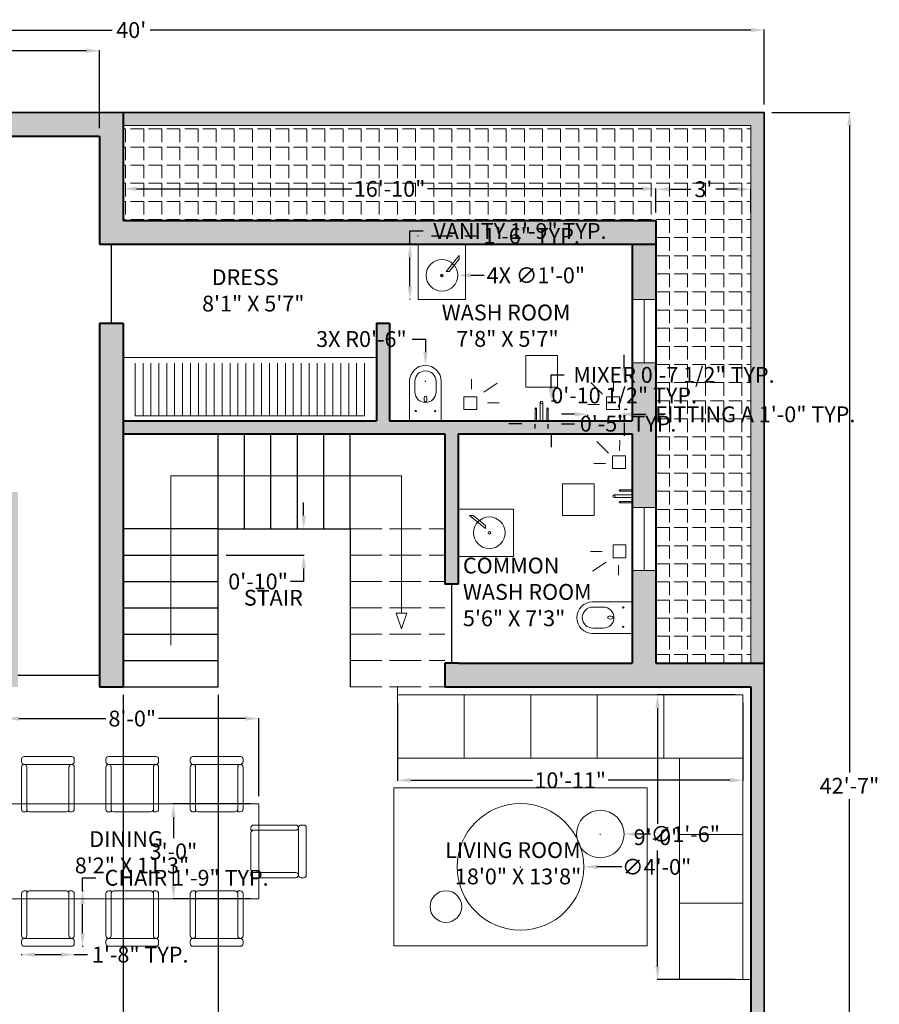
# Model space of a CAD drawing. Units: inches. Extents: x 242 to 808, y 202 to 873.
# Tile 3 of 3: x 482 to 808, y 500 to 873. Entities that reach past the tile are written whole.
import ezdxf

# ---------------------------------------------------------------- set-up
doc = ezdxf.new("R2010")
doc.units = ezdxf.units.IN
doc.header["$MEASUREMENT"] = 0
doc.linetypes.add('ACAD_ISO02W100', pattern=[15, 12, -3])
for name, color, linetype, lineweight in [('A-ANNO-DIMS', 2, 'Continuous', 18), ('A-ANNO-SYMB', 7, 'Continuous', 18), ('A-AREA-IDEN', 7, 'Continuous', 25), ('A-DOOR', 3, 'Continuous', 25), ('A-FLOR-CASE', 8, 'Continuous', 20), ('A-FLOR-FIXT', 8, 'Continuous', 18), ('A-FLOR-STRS', 7, 'Continuous', 25), ('A-FLOR-STRS-OVHD', 8, 'ACAD_ISO02W100', 18), ('A-FURN', 8, 'Continuous', 18), ('A-GLAZ', 4, 'Continuous', 18), ('A-SITE-PVMT', 8, 'Continuous', 18), ('A-SITE-PVMT-PATT', 254, 'Continuous', 13), ('A-WALL', 7, 'Continuous', 40), ('A-WALL-PATT', 30, 'Continuous', 13), ('C-PROP', 7, 'Continuous', 35)]:
    doc.layers.add(name, color=color, linetype=linetype, lineweight=lineweight)
doc.styles.get("Standard").update_dxf_attribs({"font": 'arial.ttf'})
doc.dimstyles.get("Standard").update_dxf_attribs({"dimtxt": 6, "dimasz": 5, "dimexe": 0.18, "dimexo": 3, "dimgap": 2, "dimtad": 0, "dimtih": 1, "dimtoh": 1, "dimdec": 0, "dimzin": 0, "dimdsep": 46, "dimlunit": 3, "dimtxsty": 'Standard', "dimcen": 0.09, "dimadec": 0, "dimazin": 0, "dimtfac": 1, "dimtdec": 0, "dimtofl": 0, "dimtmove": 0, "dimatfit": 3, "dimfxl": 1, "dimtolj": 1, "dimtzin": 0, "dimarcsym": 0})

# ---------------------------------------------------------------- blocks, each defined once
blk = doc.blocks.new('*U1')
blk.add_line((0, 0), (0, 20))
blk = doc.blocks.new('*U2')
at = {"layer": 'A-FLOR-CASE', "color": 0, "linetype": 'ByBlock', "lineweight": -2, "transparency": 16777216, "rotation": 90}
for p in [(883.16, 754.75), (883.16, 751.75), (883.16, 748.75), (883.16, 745.75), (883.16, 742.75), (883.16, 739.75), (883.16, 736.75), (883.16, 733.75), (883.16, 730.75), (883.16, 727.75), (883.16, 724.75), (883.16, 721.75), (883.16, 718.75), (883.16, 715.75), (883.16, 712.75), (883.16, 709.75), (883.16, 706.75), (883.16, 703.75), (883.16, 700.75), (883.16, 697.75), (883.16, 694.75), (883.16, 691.75), (883.16, 688.75), (883.16, 685.75), (883.16, 682.75), (883.16, 679.75), (883.16, 676.75), (883.16, 673.75), (883.16, 670.75), (883.16, 667.75)]:
    blk.add_blockref('*U1', p, dxfattribs=at)
blk = doc.blocks.new('*D5')
at = {"layer": 'A-ANNO-DIMS', "color": 0, "lineweight": -2, "transparency": 16777216}
for p, q in [((723.66, 800.15), (723.66, 809.17)), ((728.66, 808.99), (736.91, 808.99)), ((754.66, 808.99), (746.42, 808.99)), ((759.66, 800.15), (759.66, 809.17))]:
    blk.add_line(p, q, dxfattribs=at)
at = {"layer": 'A-ANNO-DIMS', "color": 0, "transparency": 16777216}
for points in [[(728.66, 809.82), (728.66, 808.16), (723.66, 808.99)], [(754.66, 809.82), (754.66, 808.16), (759.66, 808.99)]]:
    blk.add_solid(points, dxfattribs=at)
at = {"layer": 'Defpoints', "color": 0, "transparency": 16777216}
for p in [(759.66, 808.99), (723.66, 797.15), (759.66, 797.15)]:
    blk.add_point(p, dxfattribs=at)
at = {"layer": 'A-ANNO-DIMS', "color": 0, "transparency": 16777216, "insert": (741.66, 808.99), "char_height": 6, "attachment_point": 5}
blk.add_mtext("\\A1;3'", dxfattribs=at)
blk = doc.blocks.new('*D6')
at = {"layer": 'A-ANNO-DIMS', "color": 0, "lineweight": -2, "transparency": 16777216}
for p, q in [((521.66, 800.15), (521.66, 809.31)), ((526.66, 809.13), (608.31, 809.13)), ((718.66, 809.13), (637.02, 809.13)), ((723.66, 800.15), (723.66, 809.31))]:
    blk.add_line(p, q, dxfattribs=at)
at = {"layer": 'A-ANNO-DIMS', "color": 0, "transparency": 16777216}
for points in [[(526.66, 809.97), (526.66, 808.3), (521.66, 809.13)], [(718.66, 809.97), (718.66, 808.3), (723.66, 809.13)]]:
    blk.add_solid(points, dxfattribs=at)
at = {"layer": 'Defpoints', "color": 0, "transparency": 16777216}
for p in [(521.66, 809.13), (521.66, 797.15), (723.66, 797.15)]:
    blk.add_point(p, dxfattribs=at)
at = {"layer": 'A-ANNO-DIMS', "color": 0, "transparency": 16777216, "insert": (622.66, 809.13), "char_height": 6, "attachment_point": 5}
blk.add_mtext('\\A1;16\'-10"', dxfattribs=at)
blk = doc.blocks.new('*D7')
at = {"layer": 'A-ANNO-DIMS', "color": 0, "lineweight": -2, "transparency": 16777216}
for p, q in [((284.66, 841.15), (284.66, 869.56)), ((289.66, 869.38), (517.45, 869.38)), ((759.66, 869.38), (531.88, 869.38)), ((764.66, 841.15), (764.66, 869.56))]:
    blk.add_line(p, q, dxfattribs=at)
at = {"layer": 'A-ANNO-DIMS', "color": 0, "transparency": 16777216}
for points in [[(289.66, 870.21), (289.66, 868.54), (284.66, 869.38)], [(759.66, 870.21), (759.66, 868.54), (764.66, 869.38)]]:
    blk.add_solid(points, dxfattribs=at)
at = {"layer": 'Defpoints', "color": 0, "transparency": 16777216}
for p in [(764.66, 869.38), (284.66, 838.15), (764.66, 838.15)]:
    blk.add_point(p, dxfattribs=at)
at = {"layer": 'A-ANNO-DIMS', "color": 0, "transparency": 16777216, "insert": (524.66, 869.38), "char_height": 6, "attachment_point": 5}
blk.add_mtext("\\A1;40'", dxfattribs=at)
blk = doc.blocks.new('DINING-CHAIR')
for p, q in [((2, 18), (2, 20)), ((3, 21), (17, 21)), ((18, 21), (18, 18)), ((19, 21), (18, 21)), ((18, 20), (18, 18)), ((20, 4), (20, 20)), ((1, 0), (10, 0)), ((10, 0), (19, 0))]:
    blk.add_line(p, q)
for points in [[(0, 1), (0, 2, -0.414214), (1, 3), (1, 3, 0.414214), (2, 4), (2, 21), (1, 21, 0.414214), (0, 20), (0, 4, 0.414214), (1, 3), (19, 3)], [(18, 18), (18, 4, 0.414214), (19, 3), (19, 3, -0.414214), (20, 2), (20, 1)]]:
    blk.add_lwpolyline(points, format="xyb")
for centre, start, end in [((3, 20), 90, 180), ((17, 20), 0, 90), ((19, 20), 0, 90), ((19, 4), 270, 0), ((1, 1), 180, 270), ((19, 1), 270, 0)]:
    blk.add_arc(centre, 1, start, end)
blk = doc.blocks.new('LAVATORY-VANITY')
for p, q in [((15.59, 16.67), (10.6, 10.67)), ((11.73, 10.63), (15.59, 15.35)), ((15.59, 16.67), (15.59, 15.35)), ((10.6, 10.67), (11.73, 10.63))]:
    blk.add_line(p, q)
blk.add_lwpolyline([(0, 21), (18, 21), (18, 0), (0, 0)], close=True)
for radius in [6, 0.5]:
    blk.add_circle((8.99, 9.16), radius)
blk = doc.blocks.new('WC-PAN')
for p, q in [((0, 15), (0, 0)), ((12, 0), (12, 15)), ((2, 14.93), (2, 10.93)), ((10, 14.93), (10, 10.93))]:
    blk.add_line(p, q)
for centre, radius, start, end in [((6, 15), 6, 0, 180), ((6, 14.93), 4, 0, 180), ((6, 10.93), 4, 180, 0)]:
    blk.add_arc(centre, radius, start, end)
blk.add_ellipse((6, 8.26), major_axis=(0, 1.09), ratio=0.500408)
blk = doc.blocks.new('SHOWER-MIXER')
for p, q in [((0, 4.4), (0, 0)), ((0.5, 4.4), (0.5, 0)), ((2, 6.9), (2, 0)), ((3, 6.9), (3, 0)), ((4.5, 4.4), (4.5, 0)), ((5, 4.4), (5, 0))]:
    blk.add_line(p, q)
for centre, radius in [((0.25, 4.65), 0.25), ((2.5, 6.9), 0.5), ((4.75, 4.65), 0.25)]:
    blk.add_circle(centre, radius)
blk = doc.blocks.new('BATH-FITTING-A')
for p, q in [((5.56, 5.86), (1.12, 10.3)), ((9.72, 6.87), (9.79, 10.74)), ((4.44, 1.91), (0, 1.91))]:
    blk.add_line(p, q)
blk.add_lwpolyline([(7.09, 4.89), (11.98, 4.89), (11.98, 0), (7.09, 0)], close=True)
blk = doc.blocks.new('BATH-FITTING-B')
for p, q in [((2.85, 7.76), (2.85, 11.5)), ((7.55, 6.61), (12.62, 10.02)), ((9.01, 2.54), (13.42, 2.54))]:
    blk.add_line(p, q)
blk.add_lwpolyline([(0, 4.89), (4.89, 4.89), (4.89, 0), (0, 0)], close=True)
blk = doc.blocks.new('WIN-24IN')
blk.add_line((4.5, 24), (4.5, 0))
blk.add_lwpolyline([(0, 24), (9, 24), (9, 0), (0, 0)], close=True)
blk = doc.blocks.new('DOOR-30IN-PLAN')
blk.add_line((0, 30), (0, 0))
blk = doc.blocks.new('BATH-FITTING-12IN-SQ')
blk.add_lwpolyline([(0, 12), (12, 12), (12, 0), (0, 0)], close=True)
blk = doc.blocks.new('*D25')
at = {"layer": 'A-ANNO-DIMS', "color": 0, "lineweight": -2, "transparency": 16777216}
for p, q in [((506.21, 542.76), (506.21, 547.76)), ((506.21, 547.76), (511.21, 547.76)), ((506.06, 542.76), (506.39, 542.76)), ((506.21, 526.76), (506.21, 537.76)), ((506.06, 521.76), (506.39, 521.76))]:
    blk.add_line(p, q, dxfattribs=at)
at = {"layer": 'A-ANNO-DIMS', "color": 0, "transparency": 16777216}
for points in [[(505.38, 537.76), (507.05, 537.76), (506.21, 542.76)], [(505.38, 526.76), (507.05, 526.76), (506.21, 521.76)]]:
    blk.add_solid(points, dxfattribs=at)
at = {"layer": 'Defpoints', "color": 0, "transparency": 16777216}
for p in [(503.06, 542.76), (506.21, 542.76), (503.06, 521.76)]:
    blk.add_point(p, dxfattribs=at)
at = {"layer": 'A-ANNO-DIMS', "color": 0, "transparency": 16777216, "insert": (545.67, 547.76), "char_height": 6, "attachment_point": 5}
blk.add_mtext('\\A1;CHAIR 1\'-9" TYP.', dxfattribs=at)
blk = doc.blocks.new('*D26')
at = {"layer": 'A-ANNO-DIMS', "color": 0, "lineweight": -2, "transparency": 16777216}
for p, q in [((483.06, 518.76), (483.06, 518.43)), ((488.06, 518.61), (498.06, 518.61)), ((503.06, 518.76), (503.06, 518.43)), ((503.06, 518.61), (508.06, 518.61))]:
    blk.add_line(p, q, dxfattribs=at)
at = {"layer": 'A-ANNO-DIMS', "color": 0, "transparency": 16777216}
for points in [[(488.06, 519.44), (488.06, 517.77), (483.06, 518.61)], [(498.06, 519.44), (498.06, 517.77), (503.06, 518.61)]]:
    blk.add_solid(points, dxfattribs=at)
at = {"layer": 'Defpoints', "color": 0, "transparency": 16777216}
for p in [(483.06, 521.76), (503.06, 521.76), (503.06, 518.61)]:
    blk.add_point(p, dxfattribs=at)
at = {"layer": 'A-ANNO-DIMS', "color": 0, "transparency": 16777216, "insert": (528.07, 518.61), "char_height": 6, "attachment_point": 5}
blk.add_mtext('\\A1;1\'-8" TYP.', dxfattribs=at)
blk = doc.blocks.new('*D27')
at = {"layer": 'A-ANNO-DIMS', "color": 0, "lineweight": -2, "transparency": 16777216}
for p, q in [((630.35, 788.15), (630.35, 793.15)), ((630.35, 793.15), (635.35, 793.15)), ((630.5, 788.15), (630.17, 788.15)), ((630.35, 772.15), (630.35, 783.15)), ((630.5, 767.15), (630.17, 767.15))]:
    blk.add_line(p, q, dxfattribs=at)
at = {"layer": 'A-ANNO-DIMS', "color": 0, "transparency": 16777216}
for points in [[(629.51, 783.15), (631.18, 783.15), (630.35, 788.15)], [(629.51, 772.15), (631.18, 772.15), (630.35, 767.15)]]:
    blk.add_solid(points, dxfattribs=at)
at = {"layer": 'Defpoints', "color": 0, "transparency": 16777216}
for p in [(630.35, 788.15), (633.5, 788.15), (633.5, 767.15)]:
    blk.add_point(p, dxfattribs=at)
at = {"layer": 'A-ANNO-DIMS', "color": 0, "transparency": 16777216, "insert": (672.09, 793.15), "char_height": 6, "attachment_point": 5}
blk.add_mtext('\\A1;VANITY 1\'-9" TYP.', dxfattribs=at)
blk = doc.blocks.new('*D28')
at = {"layer": 'A-ANNO-DIMS', "color": 0, "lineweight": -2, "transparency": 16777216}
for p, q in [((633.5, 791.15), (633.5, 791.48)), ((638.5, 791.3), (646.5, 791.3)), ((651.5, 791.15), (651.5, 791.48)), ((651.5, 791.3), (656.5, 791.3))]:
    blk.add_line(p, q, dxfattribs=at)
at = {"layer": 'A-ANNO-DIMS', "color": 0, "transparency": 16777216}
for points in [[(638.5, 792.14), (638.5, 790.47), (633.5, 791.3)], [(646.5, 792.14), (646.5, 790.47), (651.5, 791.3)]]:
    blk.add_solid(points, dxfattribs=at)
at = {"layer": 'Defpoints', "color": 0, "transparency": 16777216}
for p in [(651.5, 791.3), (633.5, 788.15), (651.5, 788.15)]:
    blk.add_point(p, dxfattribs=at)
at = {"layer": 'A-ANNO-DIMS', "color": 0, "transparency": 16777216, "insert": (676.5, 791.3), "char_height": 6, "attachment_point": 5}
blk.add_mtext('\\A1;1\'-6" TYP.', dxfattribs=at)
blk = doc.blocks.new('*D31')
at = {"layer": 'A-ANNO-DIMS', "color": 0, "lineweight": -2, "transparency": 16777216}
for p, q in [((683.92, 733.55), (683.92, 738.55)), ((683.92, 738.55), (688.92, 738.55)), ((685.81, 728.55), (684.1, 728.55)), ((685.81, 721.15), (684.1, 721.15)), ((683.92, 716.15), (683.92, 711.15))]:
    blk.add_line(p, q, dxfattribs=at)
at = {"layer": 'A-ANNO-DIMS', "color": 0, "transparency": 16777216}
for points in [[(683.08, 733.55), (684.75, 733.55), (683.92, 728.55)], [(683.08, 716.15), (684.75, 716.15), (683.92, 721.15)]]:
    blk.add_solid(points, dxfattribs=at)
at = {"layer": 'Defpoints', "color": 0, "transparency": 16777216}
for p in [(682.81, 728.55), (683.92, 728.55), (682.81, 721.15)]:
    blk.add_point(p, dxfattribs=at)
at = {"layer": 'A-ANNO-DIMS', "color": 0, "transparency": 16777216, "insert": (730.5, 738.55), "char_height": 6, "attachment_point": 5}
blk.add_mtext('\\A1;MIXER 0\'-7 1/2" TYP.', dxfattribs=at)
blk = doc.blocks.new('*D32')
at = {"layer": 'A-ANNO-DIMS', "color": 0, "lineweight": -2, "transparency": 16777216}
for p, q in [((672.81, 720.04), (667.81, 720.04)), ((677.81, 718.15), (677.81, 719.86)), ((682.81, 718.15), (682.81, 719.86)), ((687.81, 720.04), (692.81, 720.04))]:
    blk.add_line(p, q, dxfattribs=at)
at = {"layer": 'A-ANNO-DIMS', "color": 0, "transparency": 16777216}
for points in [[(672.81, 720.88), (672.81, 719.21), (677.81, 720.04)], [(687.81, 720.88), (687.81, 719.21), (682.81, 720.04)]]:
    blk.add_solid(points, dxfattribs=at)
at = {"layer": 'Defpoints', "color": 0, "transparency": 16777216}
for p in [(677.81, 721.15), (682.81, 721.15), (682.81, 720.04)]:
    blk.add_point(p, dxfattribs=at)
at = {"layer": 'A-ANNO-DIMS', "color": 0, "transparency": 16777216, "insert": (713.1, 720.04), "char_height": 6, "attachment_point": 5}
blk.add_mtext('\\A1;0\'-5" TYP.', dxfattribs=at)
blk = doc.blocks.new('*D33')
at = {"layer": 'A-ANNO-DIMS', "color": 0, "lineweight": -2, "transparency": 16777216}
for p, q in [((692.82, 723.59), (687.82, 723.59)), ((697.82, 722.39), (697.82, 723.41)), ((709.8, 722.39), (709.8, 723.41)), ((714.8, 723.59), (719.8, 723.59))]:
    blk.add_line(p, q, dxfattribs=at)
at = {"layer": 'A-ANNO-DIMS', "color": 0, "transparency": 16777216}
for points in [[(692.82, 724.43), (692.82, 722.76), (697.82, 723.59)], [(714.8, 724.43), (714.8, 722.76), (709.8, 723.59)]]:
    blk.add_solid(points, dxfattribs=at)
at = {"layer": 'Defpoints', "color": 0, "transparency": 16777216}
for p in [(697.82, 725.39), (709.8, 725.39), (709.8, 723.59)]:
    blk.add_point(p, dxfattribs=at)
at = {"layer": 'A-ANNO-DIMS', "color": 0, "transparency": 16777216, "insert": (761.33, 723.59), "char_height": 6, "attachment_point": 5}
blk.add_mtext('\\A1;FITTING A 1\'-0" TYP.', dxfattribs=at)
blk = doc.blocks.new('*D34')
at = {"layer": 'A-ANNO-DIMS', "color": 0, "lineweight": -2, "transparency": 16777216}
for p, q in [((711.6, 741.13), (711.6, 746.13)), ((712.8, 736.13), (711.78, 736.13)), ((712.8, 725.39), (711.78, 725.39)), ((711.6, 720.39), (711.6, 715.39))]:
    blk.add_line(p, q, dxfattribs=at)
at = {"layer": 'A-ANNO-DIMS', "color": 0, "transparency": 16777216}
for points in [[(710.76, 741.13), (712.43, 741.13), (711.6, 736.13)], [(710.76, 720.39), (712.43, 720.39), (711.6, 725.39)]]:
    blk.add_solid(points, dxfattribs=at)
at = {"layer": 'Defpoints', "color": 0, "transparency": 16777216}
for p in [(709.8, 736.13), (711.6, 736.13), (709.8, 725.39)]:
    blk.add_point(p, dxfattribs=at)
at = {"layer": 'A-ANNO-DIMS', "color": 0, "transparency": 16777216, "insert": (711.6, 730.76), "char_height": 6, "attachment_point": 5}
blk.add_mtext('\\A1;0\'-10 1/2" TYP.', dxfattribs=at)
blk = doc.blocks.new('*D43')
at = {"layer": 'A-ANNO-DIMS', "color": 0, "lineweight": -2, "transparency": 16777216}
for p, q in [((334.66, 832.15), (334.66, 861.73)), ((339.66, 861.55), (409.31, 861.55)), ((507.66, 861.55), (438.02, 861.55)), ((512.66, 832.15), (512.66, 861.73))]:
    blk.add_line(p, q, dxfattribs=at)
at = {"layer": 'A-ANNO-DIMS', "color": 0, "transparency": 16777216}
for points in [[(339.66, 862.39), (339.66, 860.72), (334.66, 861.55)], [(507.66, 862.39), (507.66, 860.72), (512.66, 861.55)]]:
    blk.add_solid(points, dxfattribs=at)
at = {"layer": 'Defpoints', "color": 0, "transparency": 16777216}
for p in [(512.66, 861.55), (334.66, 829.15), (512.66, 829.15)]:
    blk.add_point(p, dxfattribs=at)
at = {"layer": 'A-ANNO-DIMS', "color": 0, "transparency": 16777216, "insert": (423.66, 861.55), "char_height": 6, "attachment_point": 5}
blk.add_mtext('\\A1;14\'-10"', dxfattribs=at)
blk = doc.blocks.new('*D47')
at = {"layer": 'A-ANNO-DIMS', "color": 0, "lineweight": -2, "transparency": 16777216}
for p, q in [((521.66, 617.15), (521.66, 205.57)), ((557.66, 617.15), (557.66, 205.57)), ((526.66, 205.75), (529.69, 205.75)), ((552.66, 205.75), (549.64, 205.75))]:
    blk.add_line(p, q, dxfattribs=at)
at = {"layer": 'A-ANNO-DIMS', "color": 0, "transparency": 16777216}
for points in [[(526.66, 206.59), (526.66, 204.92), (521.66, 205.75)], [(552.66, 206.59), (552.66, 204.92), (557.66, 205.75)]]:
    blk.add_solid(points, dxfattribs=at)
at = {"layer": 'Defpoints', "color": 0, "transparency": 16777216}
for p in [(521.66, 620.15), (557.66, 620.15), (557.66, 205.75)]:
    blk.add_point(p, dxfattribs=at)
at = {"layer": 'A-ANNO-DIMS', "color": 0, "transparency": 16777216, "insert": (539.66, 205.75), "char_height": 6, "attachment_point": 5}
blk.add_mtext('\\A1;3\'-0"', dxfattribs=at)
blk = doc.blocks.new('*D48')
at = {"layer": 'A-ANNO-DIMS', "color": 0, "lineweight": -2, "transparency": 16777216}
for p, q in [((767.66, 838.15), (797.24, 838.15)), ((797.06, 833.15), (797.06, 587.67)), ((797.06, 332.15), (797.06, 577.64)), ((546.66, 327.15), (797.24, 327.15))]:
    blk.add_line(p, q, dxfattribs=at)
at = {"layer": 'A-ANNO-DIMS', "color": 0, "transparency": 16777216}
for points in [[(796.23, 833.15), (797.9, 833.15), (797.06, 838.15)], [(796.23, 332.15), (797.9, 332.15), (797.06, 327.15)]]:
    blk.add_solid(points, dxfattribs=at)
at = {"layer": 'Defpoints', "color": 0, "transparency": 16777216}
for p in [(764.66, 838.15), (797.06, 838.15), (543.66, 327.15)]:
    blk.add_point(p, dxfattribs=at)
at = {"layer": 'A-ANNO-DIMS', "color": 0, "transparency": 16777216, "insert": (797.06, 582.65), "char_height": 6, "attachment_point": 5}
blk.add_mtext('\\A1;42\'-7"', dxfattribs=at)
blk = doc.blocks.new('*D50')
at = {"layer": 'A-ANNO-DIMS', "color": 0, "lineweight": -2, "transparency": 16777216}
for p, q in [((477.06, 578.76), (477.06, 608.34)), ((482.06, 608.16), (515.08, 608.16)), ((568.06, 608.16), (535.04, 608.16)), ((573.06, 578.76), (573.06, 608.34))]:
    blk.add_line(p, q, dxfattribs=at)
at = {"layer": 'A-ANNO-DIMS', "color": 0, "transparency": 16777216}
for points in [[(482.06, 608.99), (482.06, 607.32), (477.06, 608.16)], [(568.06, 608.99), (568.06, 607.32), (573.06, 608.16)]]:
    blk.add_solid(points, dxfattribs=at)
at = {"layer": 'Defpoints', "color": 0, "transparency": 16777216}
for p in [(573.06, 608.16), (477.06, 575.76), (573.06, 575.76)]:
    blk.add_point(p, dxfattribs=at)
at = {"layer": 'A-ANNO-DIMS', "color": 0, "transparency": 16777216, "insert": (525.06, 608.16), "char_height": 6, "attachment_point": 5}
blk.add_mtext('\\A1;8\'-0"', dxfattribs=at)
blk = doc.blocks.new('*D51')
at = {"layer": 'A-ANNO-DIMS', "color": 0, "lineweight": -2, "transparency": 16777216}
for p, q in [((570.06, 575.76), (540.48, 575.76)), ((540.66, 570.76), (540.66, 562.82)), ((540.66, 544.76), (540.66, 552.69)), ((570.06, 539.76), (540.48, 539.76))]:
    blk.add_line(p, q, dxfattribs=at)
at = {"layer": 'A-ANNO-DIMS', "color": 0, "transparency": 16777216}
for points in [[(539.83, 570.76), (541.5, 570.76), (540.66, 575.76)], [(539.83, 544.76), (541.5, 544.76), (540.66, 539.76)]]:
    blk.add_solid(points, dxfattribs=at)
at = {"layer": 'Defpoints', "color": 0, "transparency": 16777216}
for p in [(540.66, 575.76), (573.06, 575.76), (573.06, 539.76)]:
    blk.add_point(p, dxfattribs=at)
at = {"layer": 'A-ANNO-DIMS', "color": 0, "transparency": 16777216, "insert": (540.66, 557.76), "char_height": 6, "attachment_point": 5}
blk.add_mtext('\\A1;3\'-0"', dxfattribs=at)
blk = doc.blocks.new('*D52')
at = {"layer": 'A-ANNO-DIMS', "color": 0, "lineweight": -2, "transparency": 16777216}
for p, q in [((590.06, 685.15), (590.06, 690.15)), ((560.66, 680.15), (590.24, 680.15)), ((560.66, 670.15), (590.24, 670.15)), ((590.06, 665.15), (590.06, 660.15)), ((590.06, 660.15), (585.06, 660.15))]:
    blk.add_line(p, q, dxfattribs=at)
at = {"layer": 'A-ANNO-DIMS', "color": 0, "transparency": 16777216}
for points in [[(589.23, 685.15), (590.9, 685.15), (590.06, 680.15)], [(589.23, 665.15), (590.9, 665.15), (590.06, 670.15)]]:
    blk.add_solid(points, dxfattribs=at)
at = {"layer": 'Defpoints', "color": 0, "transparency": 16777216}
for p in [(557.66, 680.15), (557.66, 670.15), (590.06, 670.15)]:
    blk.add_point(p, dxfattribs=at)
at = {"layer": 'A-ANNO-DIMS', "color": 0, "transparency": 16777216, "insert": (572.76, 660.15), "char_height": 6, "attachment_point": 5}
blk.add_mtext('\\A1;0\'-10"', dxfattribs=at)
blk = doc.blocks.new('*D56')
at = {"layer": 'A-ANNO-DIMS', "color": 0, "lineweight": -2, "transparency": 16777216}
for p, q in [((625.66, 614.15), (625.66, 584.57)), ((756.66, 614.15), (756.66, 584.57)), ((630.66, 584.75), (676.81, 584.75)), ((751.66, 584.75), (705.52, 584.75))]:
    blk.add_line(p, q, dxfattribs=at)
at = {"layer": 'A-ANNO-DIMS', "color": 0, "transparency": 16777216}
for points in [[(630.66, 585.59), (630.66, 583.92), (625.66, 584.75)], [(751.66, 585.59), (751.66, 583.92), (756.66, 584.75)]]:
    blk.add_solid(points, dxfattribs=at)
at = {"layer": 'Defpoints', "color": 0, "transparency": 16777216}
for p in [(625.66, 617.15), (756.66, 617.15), (625.66, 584.75)]:
    blk.add_point(p, dxfattribs=at)
at = {"layer": 'A-ANNO-DIMS', "color": 0, "transparency": 16777216, "insert": (691.16, 584.75), "char_height": 6, "attachment_point": 5}
blk.add_mtext('\\A1;10\'-11"', dxfattribs=at)
blk = doc.blocks.new('*D57')
at = {"layer": 'A-ANNO-DIMS', "color": 0, "lineweight": -2, "transparency": 16777216}
for p, q in [((753.66, 617.15), (724.08, 617.15)), ((724.26, 612.15), (724.26, 568.22)), ((724.26, 514.15), (724.26, 558.09)), ((753.66, 509.15), (724.08, 509.15))]:
    blk.add_line(p, q, dxfattribs=at)
at = {"layer": 'A-ANNO-DIMS', "color": 0, "transparency": 16777216}
for points in [[(723.43, 612.15), (725.1, 612.15), (724.26, 617.15)], [(723.43, 514.15), (725.1, 514.15), (724.26, 509.15)]]:
    blk.add_solid(points, dxfattribs=at)
at = {"layer": 'Defpoints', "color": 0, "transparency": 16777216}
for p in [(724.26, 617.15), (756.66, 617.15), (756.66, 509.15)]:
    blk.add_point(p, dxfattribs=at)
at = {"layer": 'A-ANNO-DIMS', "color": 0, "transparency": 16777216, "insert": (724.26, 563.15), "char_height": 6, "attachment_point": 5}
blk.add_mtext('\\A1;9\'-0"', dxfattribs=at)
blk = doc.blocks.new('*D58')
at = {"layer": 'A-ANNO-DIMS', "color": 0, "lineweight": -2, "transparency": 16777216}
for p, q in [((672.19, 551.88), (672.37, 551.88)), ((672.28, 551.79), (672.28, 551.97)), ((710.68, 551.88), (701.28, 551.88))]:
    blk.add_line(p, q, dxfattribs=at)
at = {"layer": 'A-ANNO-DIMS', "color": 0, "transparency": 16777216}
blk.add_solid([(701.28, 552.72), (701.28, 551.05), (696.28, 551.88)], dxfattribs=at)
at = {"layer": 'Defpoints', "color": 0, "transparency": 16777216}
for p in [(648.28, 551.88), (696.28, 551.88)]:
    blk.add_point(p, dxfattribs=at)
at = {"layer": 'A-ANNO-DIMS', "color": 0, "transparency": 16777216, "insert": (723.91, 551.88), "char_height": 6, "attachment_point": 5}
blk.add_mtext('\\A1;∅4\'-0"', dxfattribs=at)
blk = doc.blocks.new('*D59')
at = {"layer": 'A-ANNO-DIMS', "color": 0, "lineweight": -2, "transparency": 16777216}
for p, q in [((702.48, 564.33), (702.66, 564.33)), ((702.57, 564.24), (702.57, 564.42)), ((721.57, 564.33), (716.57, 564.33))]:
    blk.add_line(p, q, dxfattribs=at)
at = {"layer": 'A-ANNO-DIMS', "color": 0, "transparency": 16777216}
blk.add_solid([(716.57, 565.16), (716.57, 563.5), (711.57, 564.33)], dxfattribs=at)
at = {"layer": 'Defpoints', "color": 0, "transparency": 16777216}
for p in [(693.57, 564.33), (711.57, 564.33)]:
    blk.add_point(p, dxfattribs=at)
at = {"layer": 'A-ANNO-DIMS', "color": 0, "transparency": 16777216, "insert": (734.81, 564.33), "char_height": 6, "attachment_point": 5}
blk.add_mtext('\\A1;∅1\'-6"', dxfattribs=at)
blk = doc.blocks.new('*D60')
at = {"layer": 'A-ANNO-DIMS', "color": 0, "lineweight": -2, "transparency": 16777216}
for p, q in [((642.39, 776.31), (642.57, 776.31)), ((642.48, 776.22), (642.48, 776.4)), ((658.48, 776.31), (653.48, 776.31))]:
    blk.add_line(p, q, dxfattribs=at)
at = {"layer": 'A-ANNO-DIMS', "color": 0, "transparency": 16777216}
blk.add_solid([(653.48, 777.15), (653.48, 775.48), (648.48, 776.31)], dxfattribs=at)
at = {"layer": 'Defpoints', "color": 0, "transparency": 16777216}
for p in [(636.48, 776.31), (648.48, 776.31)]:
    blk.add_point(p, dxfattribs=at)
at = {"layer": 'A-ANNO-DIMS', "color": 0, "transparency": 16777216, "insert": (678.13, 776.31), "char_height": 6, "attachment_point": 5}
blk.add_mtext('\\A1;4X ∅1\'-0"', dxfattribs=at)
blk = doc.blocks.new('*D61')
at = {"layer": 'A-ANNO-DIMS', "color": 0, "lineweight": -2, "transparency": 16777216}
for p, q in [((631.25, 752.15), (636.25, 752.15)), ((636.25, 752.15), (636.25, 747.15)), ((636.16, 736.15), (636.34, 736.15)), ((636.25, 736.06), (636.25, 736.24))]:
    blk.add_line(p, q, dxfattribs=at)
at = {"layer": 'A-ANNO-DIMS', "color": 0, "transparency": 16777216}
blk.add_solid([(637.08, 747.15), (635.41, 747.15), (636.25, 742.15)], dxfattribs=at)
at = {"layer": 'Defpoints', "color": 0, "transparency": 16777216}
for p in [(636.25, 742.15), (636.25, 736.15)]:
    blk.add_point(p, dxfattribs=at)
at = {"layer": 'A-ANNO-DIMS', "color": 0, "transparency": 16777216, "insert": (611.96, 752.15), "char_height": 6, "attachment_point": 5}
blk.add_mtext('\\A1;3X R0\'-6"', dxfattribs=at)

msp = doc.modelspace()

# ---------------------------------------------------------------- hatches: boundary and pattern name
at = {"layer": 'A-SITE-PVMT-PATT'}
h = msp.add_hatch(dxfattribs=at)
h.set_pattern_fill('ANGLE', color=256, scale=25, angle=180)
h.set_pattern_definition([(180, (0, 0), (-8e-16, -6.875), [5, -1.875]), (270, (0, 0), (6.875, -1e-15), [5, -1.875])])
h.paths.add_polyline_path([(759.66, 833.15), (521.66, 833.15), (521.66, 797.15), (723.66, 797.15), (723.66, 629.15), (759.66, 629.15)])
h.paths.add_polyline_path([(737.05, 802.77), (746.32, 802.77), (746.32, 815.13), (737.05, 815.13)], flags=24)
h.paths.add_polyline_path([(607.9, 802.91), (636.91, 802.91), (636.91, 815.27), (607.9, 815.27)], flags=24)
at = {"layer": 'A-WALL-PATT'}
h = msp.add_hatch(color=256, dxfattribs=at)
h.dxf.hatch_style = 1
h.paths.add_polyline_path([(521.66, 838.15), (325.66, 838.15), (325.66, 789.05), (334.66, 789.05), (334.66, 829.15), (512.66, 829.15), (512.66, 788.15), (714.66, 788.15), (723.66, 788.15), (723.66, 797.15), (521.66, 797.15)])
h.paths.add_polyline_path([(764.66, 838.15), (521.66, 838.15), (521.66, 833.15), (759.66, 833.15), (759.66, 629.15), (764.66, 629.15)])
h.paths.add_polyline_path([(723.66, 788.15), (714.66, 788.15), (714.66, 767.17), (723.66, 767.17)], flags=17)
h.paths.add_polyline_path([(723.66, 743.17), (714.66, 743.17), (714.66, 721.15), (622.66, 721.15), (622.66, 758.15), (617.66, 758.15), (617.66, 721.15), (521.66, 721.15), (521.66, 716.15), (643.66, 716.15), (643.66, 659.15), (648.66, 659.15), (648.66, 716.15), (714.66, 716.15), (714.66, 688.28), (723.66, 688.28)], flags=17)
h.paths.add_polyline_path([(764.66, 629.15), (759.66, 629.15), (723.66, 629.15), (723.66, 664.28), (714.66, 664.28), (714.66, 629.15), (648.66, 629.15), (643.66, 629.15), (643.66, 620.15), (759.66, 620.15), (759.66, 403.15), (759.66, 398.15), (759.66, 238.15), (764.66, 238.15)])
h.paths.add_polyline_path([(521.66, 758.15), (512.66, 758.15), (512.66, 620.15), (521.66, 620.15)])
h.paths.add_polyline_path([(481.66, 694.15), (334.66, 694.15), (334.66, 689.15), (476.66, 689.15), (476.66, 629.15), (481.66, 629.15)])
h.paths.add_polyline_path([(334.66, 741.05), (325.66, 741.05), (325.66, 675.31), (334.66, 675.31), (334.66, 689.15), (334.66, 694.15)], flags=17)
h.paths.add_polyline_path([(334.66, 651.31), (325.66, 651.31), (325.66, 629.15), (289.66, 629.15), (289.66, 838.15), (284.66, 838.15), (284.66, 620.15), (293.66, 620.15), (334.66, 620.15)])
h.paths.add_polyline_path([(293.66, 620.15), (284.66, 620.15), (284.66, 485.15), (293.66, 485.15)])
h.paths.add_polyline_path([(307.66, 485.15), (293.66, 485.15), (284.66, 485.15), (284.66, 238.15), (615.66, 238.15), (615.66, 243.15), (289.66, 243.15), (289.66, 480.15), (307.66, 480.15)])
h.paths.add_polyline_path([(373.66, 485.15), (355.66, 485.15), (355.66, 480.15), (373.66, 480.15)], flags=17)
h.paths.add_polyline_path([(445.66, 620.15), (440.66, 620.15), (440.66, 485.15), (373.66, 485.15), (373.66, 480.15), (373.66, 415.15), (410.66, 415.15), (410.66, 420.15), (378.66, 420.15), (378.66, 480.15), (440.66, 480.15), (440.66, 415.15), (445.66, 415.15)])
h.paths.add_polyline_path([(472.95, 336.15), (444.15, 336.15), (444.15, 327.15), (472.95, 327.15)], flags=17)
h.paths.add_polyline_path([(543.66, 485.15), (481.66, 485.15), (481.66, 480.15), (534.66, 480.15), (534.66, 336.15), (520.95, 336.15), (520.95, 327.15), (543.66, 327.15)], flags=17)
h.paths.add_polyline_path([(699.66, 456.15), (649.16, 456.15), (649.16, 451.15), (694.66, 451.15), (694.66, 398.15), (759.66, 398.15), (759.66, 403.15), (699.66, 403.15)], flags=17)
h.paths.add_polyline_path([(481.66, 629.15), (476.66, 629.15), (364.66, 629.15), (364.66, 620.15), (481.66, 620.15)])

# ---------------------------------------------------------------- linework, layer by layer
at = {"layer": 'A-ANNO-SYMB'}
for p, q in [((539.66, 640.15), (539.66, 700.21)), ((539.66, 700.21), (627.17, 700.21)), ((627.17, 700.21), (627.17, 648.16)), ((629.17, 648.16), (625.17, 648.16)), ((625.17, 648.16), (627.17, 642.16)), ((627.17, 642.16), (629.17, 648.16)), ((539.66, 640.15), (539.66, 635.98))]:
    msp.add_line(p, q, dxfattribs=at)
at = {"layer": 'A-DOOR'}
msp.add_line((481.66, 624.65), (512.66, 624.65), dxfattribs=at)
at = {"layer": 'A-FLOR-CASE'}
for p, q in [((521.66, 745.15), (617.66, 745.15)), ((613.14, 723.05), (526.14, 723.05))]:
    msp.add_line(p, q, dxfattribs=at)
at = {"layer": 'A-FLOR-FIXT'}
for centre in [(632.56, 724.85), (639.94, 724.85), (711.25, 650.35), (711.25, 642.96)]:
    msp.add_circle(centre, 0.25, dxfattribs=at)
at = {"layer": 'A-FLOR-STRS'}
for p, q in [((557.66, 680.15), (557.66, 716.15)), ((567.66, 680.15), (567.66, 716.15)), ((577.66, 680.15), (577.66, 716.15)), ((587.66, 680.15), (587.66, 716.15)), ((597.66, 680.15), (597.66, 716.15)), ((607.66, 680.15), (607.66, 716.15)), ((557.66, 680.15), (521.66, 680.15)), ((557.66, 620.15), (557.66, 680.15)), ((557.66, 680.15), (607.66, 680.15)), ((607.66, 680.15), (607.66, 620.15)), ((521.66, 670.15), (557.66, 670.15)), ((521.66, 660.15), (557.66, 660.15)), ((521.66, 650.15), (557.66, 650.15)), ((521.66, 640.15), (557.66, 640.15)), ((521.66, 630.15), (557.66, 630.15)), ((521.66, 620.15), (557.66, 620.15))]:
    msp.add_line(p, q, dxfattribs=at)
at = {"layer": 'A-FLOR-STRS-OVHD'}
for p, q in [((607.66, 680.15), (643.66, 680.15)), ((607.66, 670.15), (643.66, 670.15)), ((607.66, 660.15), (643.66, 660.15)), ((607.66, 650.15), (643.66, 650.15)), ((607.66, 640.15), (643.66, 640.15)), ((607.66, 630.15), (643.66, 630.15)), ((607.66, 620.15), (643.66, 620.15))]:
    msp.add_line(p, q, dxfattribs=at)
at = {"layer": 'A-FURN'}
for p, q in [((625.66, 620.15), (625.66, 593.15)), ((625.66, 617.15), (756.66, 617.15)), ((650.91, 593.15), (650.91, 617.15)), ((676.16, 593.15), (676.16, 617.15)), ((701.41, 593.15), (701.41, 617.15)), ((726.66, 593.15), (726.66, 617.15)), ((756.66, 617.15), (756.66, 509.15)), ((625.66, 593.15), (732.66, 593.15)), ((732.66, 593.15), (732.66, 509.15)), ((732.66, 593.15), (756.66, 593.15)), ((570.06, 566.76), (570.06, 565.76)), ((570.06, 565.76), (573.06, 565.76)), ((570.06, 550.76), (570.06, 564.76)), ((587.06, 567.76), (571.06, 567.76)), ((571.06, 565.76), (573.06, 565.76)), ((591.06, 557.76), (591.06, 566.76)), ((732.66, 564.15), (756.66, 564.15)), ((591.06, 548.76), (591.06, 557.76)), ((573.06, 549.76), (571.06, 549.76)), ((732.66, 538.15), (756.66, 538.15)), ((732.66, 509.15), (759.66, 509.15))]:
    msp.add_line(p, q, dxfattribs=at)
for points in [[(624.28, 581.88), (720.28, 581.88), (720.28, 521.88), (624.28, 521.88)], [(477.06, 575.76), (573.06, 575.76), (573.06, 539.76), (477.06, 539.76)]]:
    msp.add_lwpolyline(points, close=True, dxfattribs=at)
for points in [[(590.06, 547.76), (589.06, 547.76, -0.414214), (588.06, 548.76), (588.06, 548.76, 0.414214), (587.06, 549.76), (570.06, 549.76), (570.06, 548.76, 0.414214), (571.06, 547.76), (587.06, 547.76, 0.414214), (588.06, 548.76), (588.06, 566.76)], [(573.06, 565.76), (587.06, 565.76, 0.414214), (588.06, 566.76), (588.06, 566.76, -0.414214), (589.06, 567.76), (590.06, 567.76)]]:
    msp.add_lwpolyline(points, format="xyb", dxfattribs=at)
for centre, radius in [((672.28, 551.88), 24), ((702.57, 564.33), 9), ((643.99, 536.84), 6)]:
    msp.add_circle(centre, radius, dxfattribs=at)
for centre, start, end in [((571.06, 566.76), 90, 180), ((571.06, 564.76), 90, 180), ((587.06, 566.76), 0, 90), ((590.06, 566.76), 0, 90), ((571.06, 550.76), 180, 270), ((590.06, 548.76), 270, 0)]:
    msp.add_arc(centre, 1, start, end, dxfattribs=at)
at = {"layer": 'A-SITE-PVMT'}
for p, q in [((521.66, 833.15), (759.66, 833.15)), ((759.66, 833.15), (759.66, 629.15))]:
    msp.add_line(p, q, dxfattribs=at)
at = {"layer": 'A-WALL'}
for p, q in [((521.66, 838.15), (521.66, 797.15)), ((334.66, 829.15), (512.66, 829.15)), ((512.66, 829.15), (512.66, 788.15)), ((521.66, 797.15), (723.66, 797.15)), ((723.66, 797.15), (723.66, 629.15)), ((512.66, 788.15), (714.66, 788.15)), ((521.66, 788.15), (617.66, 788.15)), ((714.66, 788.15), (714.66, 721.15)), ((714.66, 788.15), (723.66, 788.15)), ((512.66, 758.15), (521.66, 758.15)), ((512.66, 758.15), (512.66, 620.15)), ((521.66, 758.15), (521.66, 620.15)), ((617.66, 758.15), (617.66, 721.15)), ((617.66, 758.15), (622.66, 758.15)), ((622.66, 758.15), (622.66, 721.15)), ((521.66, 721.15), (617.66, 721.15)), ((622.66, 721.15), (714.66, 721.15)), ((521.66, 716.15), (643.66, 716.15)), ((643.66, 716.15), (643.66, 659.15)), ((648.66, 716.15), (648.66, 659.15)), ((648.66, 716.15), (714.66, 716.15)), ((714.66, 716.15), (714.66, 629.15)), ((648.66, 659.15), (643.66, 659.15)), ((648.66, 629.15), (643.66, 629.15)), ((643.66, 629.15), (643.66, 620.15)), ((648.66, 629.15), (714.66, 629.15)), ((723.66, 629.15), (759.66, 629.15)), ((759.66, 629.15), (764.66, 629.15)), ((512.66, 620.15), (521.66, 620.15)), ((643.66, 620.15), (759.66, 620.15)), ((759.66, 620.15), (759.66, 403.15))]:
    msp.add_line(p, q, dxfattribs=at)
at = {"layer": 'C-PROP'}
for p, q in [((284.66, 838.15), (764.66, 838.15)), ((764.66, 838.15), (764.66, 238.15))]:
    msp.add_line(p, q, dxfattribs=at)

# ---------------------------------------------------------------- block references
at = {"layer": 'A-DOOR', "rotation": 180}
msp.add_blockref('DOOR-30IN-PLAN', (517.16, 788.15), dxfattribs=at)
at = {"layer": 'A-DOOR'}
msp.add_blockref('DOOR-30IN-PLAN', (646.16, 629.15), dxfattribs=at)
at = {"layer": 'A-FLOR-CASE', "rotation": 270}
msp.add_blockref('*U2', (-141.62, 1606.2), dxfattribs=at)
at = {"layer": 'A-FLOR-FIXT'}
for name, p in [('LAVATORY-VANITY', (633.5, 767.15)), ('BATH-FITTING-12IN-SQ', (674.31, 733.95)), ('WC-PAN', (630.25, 721.15)), ('BATH-FITTING-B', (650.82, 725.39)), ('BATH-FITTING-A', (697.82, 725.39)), ('SHOWER-MIXER', (677.81, 721.15)), ('BATH-FITTING-A', (700.12, 703.01))]:
    msp.add_blockref(name, p, dxfattribs=at)
for name, p, rotation in [('BATH-FITTING-12IN-SQ', (700.28, 685.18), 90.00000000000045), ('SHOWER-MIXER', (714.66, 689.99), 89.99999999999912), ('LAVATORY-VANITY', (669.66, 669.65), 90.00000000000028), ('BATH-FITTING-B', (712.28, 674.07), 180), ('WC-PAN', (714.66, 640.46), 89.9999999999989)]:
    msp.add_blockref(name, p, dxfattribs=dict(at, rotation=rotation))
at = {"layer": 'A-FURN', "extrusion": (0, 0, -1), "zscale": -1, "rotation": 180}
for p in [(-483.06, 593.76), (-515.06, 593.76), (-547.06, 593.76)]:
    msp.add_blockref('DINING-CHAIR', p, dxfattribs=at)
at = {"layer": 'A-FURN'}
for p in [(483.06, 521.76), (515.06, 521.76), (547.06, 521.76)]:
    msp.add_blockref('DINING-CHAIR', p, dxfattribs=at)
at = {"layer": 'A-GLAZ'}
for p in [(714.66, 743.17), (714.66, 664.28)]:
    msp.add_blockref('WIN-24IN', p, dxfattribs=at)

# ---------------------------------------------------------------- texts
at = {"layer": 'A-AREA-IDEN', "char_height": 6, "attachment_point": 1}
for s, insert in [('      DRESS\\P    8\'1" X 5\'7"', (544.19, 778.61)), ('WASH ROOM \\P   7\'8" X 5\'7"', (642.42, 765.22)), ('COMMON\\PWASH ROOM\\P5\'6" X 7\'3"', (650.46, 669.21)), ('STAIR', (567.37, 657)), ('   DINING \\P8\'2" X 11\'3"', (503.26, 565.43)), ('  LIVING ROOM\\P    18\'0" X 13\'8"', (640.09, 561.26))]:
    msp.add_mtext_dynamic_manual_height_columns(s, width=78.0144, gutter_width=1, heights=[0], dxfattribs=dict(at, insert=insert))

# ---------------------------------------------------------------- dimensions: what is measured, and where the dimension line sits
at = {"layer": 'A-ANNO-DIMS'}
for base, p1, p2, override, picture, middle in [((764.66, 869.38), (284.66, 838.15), (764.66, 838.15), {"dimclrd": 0, "dimclre": 0, "dimclrt": 0}, '*D7', (524.66, 869.38)), ((512.66, 861.55), (334.66, 829.15), (512.66, 829.15), {"dimdec": 1, "dimlfac": 1, "dimrnd": 0, "dimzin": 1, "dimdsep": 46, "dimlunit": 4, "dimfrac": 2}, '*D43', (423.66, 861.55)), ((521.66, 809.13), (723.66, 797.15), (521.66, 797.15), {"dimclrd": 0, "dimclre": 0, "dimclrt": 0}, '*D6', (622.66, 809.13)), ((759.66, 808.99), (723.66, 797.15), (759.66, 797.15), {"dimclrd": 0, "dimclre": 0, "dimclrt": 0}, '*D5', (741.66, 808.99)), ((557.66, 205.75), (521.66, 620.15), (557.66, 620.15), {"dimdec": 1, "dimlfac": 1, "dimrnd": 0, "dimzin": 1, "dimdsep": 46, "dimlunit": 4, "dimfrac": 2}, '*D47', (539.66, 205.75)), ((573.06, 608.16), (477.06, 575.76), (573.06, 575.76), {"dimdec": 1, "dimlfac": 1, "dimrnd": 0, "dimzin": 1, "dimdsep": 46, "dimlunit": 4, "dimfrac": 2}, '*D50', (525.06, 608.16))]:
    dim = msp.add_linear_dim(base=base, p1=p1, p2=p2, dimstyle='Standard', override=override, dxfattribs=at)
    dim.commit()
    dim.dimension.update_dxf_attribs({"geometry": picture, "text_midpoint": middle})
for base, p1, p2, angle, picture, middle in [((797.06, 838.15), (543.66, 327.15), (764.66, 838.15), 90, '*D48', (797.06, 582.65)), ((590.06, 670.15), (557.66, 680.15), (557.66, 670.15), 270, '*D52', (572.76, 660.15)), ((625.66, 584.75), (756.66, 617.15), (625.66, 617.15), 180, '*D56', (691.16, 584.75)), ((724.26, 617.15), (756.66, 509.15), (756.66, 617.15), 90, '*D57', (724.26, 563.15)), ((540.66, 575.76), (573.06, 539.76), (573.06, 575.76), 90, '*D51', (540.66, 557.76))]:
    dim = msp.add_linear_dim(base=base, p1=p1, p2=p2, angle=angle, dimstyle='Standard', override={"dimdec": 1, "dimlfac": 1, "dimrnd": 0, "dimzin": 1, "dimdsep": 46, "dimlunit": 4, "dimfrac": 2}, dxfattribs=at)
    dim.commit()
    dim.dimension.update_dxf_attribs({"geometry": picture, "text_midpoint": middle})
for base, p1, p2, text, picture, middle in [((630.35, 788.15), (633.5, 767.15), (633.5, 788.15), 'VANITY <> TYP.', '*D27', (672.09, 793.15)), ((683.92, 728.55), (682.81, 721.15), (682.81, 728.55), 'MIXER <> TYP.', '*D31', (730.5, 738.55)), ((711.6, 736.13), (709.8, 725.39), (709.8, 736.13), '<> TYP.', '*D34', (711.6, 730.76)), ((506.21, 542.76), (503.06, 521.76), (503.06, 542.76), 'CHAIR <> TYP.', '*D25', (545.67, 547.76))]:
    dim = msp.add_linear_dim(base=base, p1=p1, p2=p2, angle=90, text=text, dimstyle='Standard', override={"dimdec": 1, "dimlfac": 1, "dimrnd": 0, "dimzin": 1, "dimdsep": 46, "dimlunit": 4, "dimfrac": 2}, dxfattribs=at)
    dim.commit()
    dim.dimension.update_dxf_attribs({"geometry": picture, "text_midpoint": middle})
for base, p1, p2, text, picture, middle in [((651.5, 791.3), (633.5, 788.15), (651.5, 788.15), '<> TYP.', '*D28', (676.5, 791.3)), ((709.8, 723.59), (697.82, 725.39), (709.8, 725.39), 'FITTING A <> TYP.', '*D33', (761.33, 723.59)), ((682.81, 720.04), (677.81, 721.15), (682.81, 721.15), '<> TYP.', '*D32', (713.1, 720.04)), ((503.06, 518.61), (483.06, 521.76), (503.06, 521.76), '<> TYP.', '*D26', (528.07, 518.61))]:
    dim = msp.add_linear_dim(base=base, p1=p1, p2=p2, text=text, dimstyle='Standard', override={"dimdec": 1, "dimlfac": 1, "dimrnd": 0, "dimzin": 1, "dimdsep": 46, "dimlunit": 4, "dimfrac": 2}, dxfattribs=at)
    dim.commit()
    dim.dimension.update_dxf_attribs({"geometry": picture, "text_midpoint": middle})
dim = msp.add_diameter_dim_2p(p1=(636.48, 776.31), p2=(648.48, 776.31), text='4X <>', dimstyle='Standard', override={"dimdec": 1, "dimlfac": 1, "dimrnd": 0, "dimzin": 1, "dimdsep": 46, "dimlunit": 4, "dimfrac": 2}, dxfattribs=at)
dim.commit()
dim.dimension.update_dxf_attribs({"geometry": '*D60', "text_midpoint": (658.48, 776.31), "dimtype": 163})
dim = msp.add_radius_dim(center=(636.25, 736.15), mpoint=(636.25, 742.15), text='3X <>', dimstyle='Standard', override={"dimdec": 1, "dimlfac": 1, "dimrnd": 0, "dimzin": 1, "dimdsep": 46, "dimlunit": 4, "dimfrac": 2}, dxfattribs=at)
dim.commit()
dim.dimension.update_dxf_attribs({"geometry": '*D61', "text_midpoint": (611.96, 752.15)})
for p1, p2, picture, middle in [((693.57, 564.33), (711.57, 564.33), '*D59', (721.57, 564.33)), ((648.28, 551.88), (696.28, 551.88), '*D58', (710.68, 551.88))]:
    dim = msp.add_diameter_dim_2p(p1=p1, p2=p2, dimstyle='Standard', override={"dimdec": 1, "dimlfac": 1, "dimrnd": 0, "dimzin": 1, "dimdsep": 46, "dimlunit": 4, "dimfrac": 2}, dxfattribs=at)
    dim.commit()
    dim.dimension.update_dxf_attribs({"geometry": picture, "text_midpoint": middle, "dimtype": 163})

doc.saveas('drawing.dxf')
